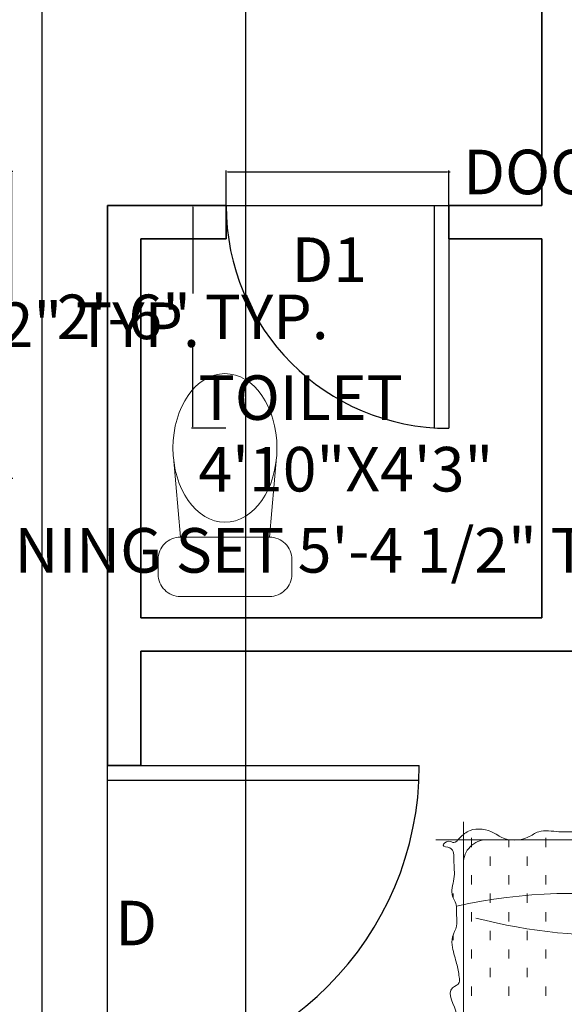
# Model space of a CAD drawing. Units: inches. Extents: x -26 to 575, y -18 to 513.
# Tile 8 of 28: x 122 to 196, y 191 to 324. Entities that reach past the tile are written whole.
import ezdxf

# ---------------------------------------------------------------- set-up
doc = ezdxf.new("R2010")
doc.units = ezdxf.units.IN
doc.header["$MEASUREMENT"] = 0
for name, color, linetype, lineweight in [('A-ANNO-DIMS', 2, 'Continuous', 18), ('A-ANNO-TEXT', 7, 'Continuous', 18), ('A-AREA-IDEN', 7, 'Continuous', 18), ('A-DOOR', 3, 'Continuous', 25), ('A-FLOR-FIXT', 9, 'Continuous', 18), ('A-WALL', 7, 'Continuous', 35), ('Furniture', 8, 'Continuous', 15)]:
    doc.layers.add(name, color=color, linetype=linetype, lineweight=lineweight)
doc.styles.get("Standard").update_dxf_attribs({"font": 'arial.ttf', "height": 6})
doc.dimstyles.get("Standard").update_dxf_attribs({"dimtxt": 6, "dimasz": 0.18, "dimexe": 0.18, "dimexo": 0.0625, "dimgap": 0.09, "dimtad": 0, "dimtih": 1, "dimtoh": 1, "dimzin": 0, "dimdsep": 46, "dimlunit": 3, "dimtxsty": 'Standard', "dimcen": 0.09, "dimadec": 0, "dimazin": 0, "dimtfac": 1, "dimtofl": 0, "dimtmove": 0, "dimatfit": 3, "dimfxl": 1, "dimtolj": 1, "dimtzin": 0, "dimarcsym": 0})

# ---------------------------------------------------------------- blocks, each defined once
blk = doc.blocks.new('BED-DOUBLE-WITH-NIGHTSTANDS')
for p, q in [((81.88, 42.36), (81.88, 0)), ((70.77, 22.17), (70.77, 23.42)), ((75.77, 22.17), (75.77, 23.42)), ((80.77, 22.17), (80.77, 23.42)), ((73.27, 19.67), (73.27, 20.92)), ((78.27, 19.67), (78.27, 20.92)), ((70.77, 17.17), (70.77, 18.42)), ((75.77, 17.17), (75.77, 18.42)), ((80.77, 17.17), (80.77, 18.42)), ((73.27, 14.67), (73.27, 15.92)), ((78.27, 14.67), (78.27, 15.92)), ((83.27, 15.26), (83.27, 15.92)), ((70.77, 12.17), (70.77, 13.42)), ((75.77, 12.17), (75.77, 13.42)), ((80.77, 12.17), (80.77, 13.42)), ((73.27, 9.67), (73.27, 10.92)), ((78.27, 9.67), (78.27, 10.92)), ((83.27, 9.67), (83.27, 10.2)), ((70.77, 7.17), (70.77, 8.42)), ((75.77, 7.17), (75.77, 8.42)), ((80.77, 7.17), (80.77, 8.42)), ((73.27, 4.67), (73.27, 5.92)), ((78.27, 4.67), (78.27, 5.92)), ((70.77, 2.17), (70.77, 3.42)), ((75.77, 2.41), (75.77, 3.42)), ((80.77, 2.17), (80.77, 3.42)), ((85.58, 2.43), (23.7, 2.43))]:
    blk.add_line(p, q)
for centre, radius, start, end in [((66.97, 82.6), 72.97, 239.8126, 282.5472), ((61.48, -60.53), 75.85, 75.7143, 109.4459), ((78.73, 5.58), 3.15, 270, 0)]:
    blk.add_arc(centre, radius, start, end)
blk.add_open_spline([(82.95, 38.85), (82.91, 38.17), (82.85, 36.97), (81.76, 35.43), (82.66, 33.92), (82.17, 32.16), (83.17, 30.81), (83.54, 28.6), (81.84, 26.13), (84.59, 22.62), (82.27, 21.86), (82.5, 20.48), (82.77, 18.98), (83.36, 17.21), (83.5, 15.41), (82.61, 14.09), (82.87, 12.46), (82.71, 11.04), (83.72, 9.61), (82.91, 7.55), (83.23, 5.58), (83.08, 3.39), (85.08, 3.34), (83.88, 2.36), (83.09, 3.04), (82.19, 1.93), (80.71, 0.69), (78.27, 1.05), (76.16, 2.63), (73.68, 2.58), (71.48, 0.95), (69.05, 1.47), (65.15, 1.19), (60.81, 2), (56.05, 2.59), (52.45, 0.27), (49.19, 1.51), (46.12, 1.7), (37.69, 3.67), (31.84, 3.18), (20.44, -0.09), (22.21, 3.75), (19.18, -0.44), (22.91, 0.39), (27.14, 0.63), (21.63, 1.85), (19.68, 4.27), (19.87, 11.16), (24.26, 3.84), (20.3, 10.76), (23.26, 12.85), (24.33, 17.43), (16.78, 17.59), (25.96, 19.23), (16.2, 20.68), (24.67, 22.01), (20.04, 24.96), (24.6, 28.15), (20.03, 29.6), (23.48, 31.6), (22.43, 34.55), (22.92, 41.18), (22.85, 37.06), (22.83, 35.35)], degree=3, knots=[0, 0, 0, 0, 2.033881, 3.581387, 5.07489, 6.704853, 8.655612, 9.757262, 13.24098, 16.903694, 18.063816, 18.788243, 20.635227, 22.875483, 24.324336, 25.871843, 27.320698, 29.140811, 29.950855, 32.312207, 34.847704, 36.565952, 37.541804, 38.447727, 39.194923, 40.100844, 41.912688, 45.194843, 46.251388, 49.875946, 51.496686, 54.215105, 56.7523, 63.316606, 67.484853, 70.581422, 75.324573, 76.965649, 79.915763, 100.671038, 102.483321, 104.317501, 106.523635, 109.038061, 111.571263, 115.809372, 117.667229, 122.411431, 125.445794, 129.976907, 132.758854, 136.424739, 139.918708, 143.481583, 147.135325, 151.002466, 153.252794, 157.23352, 159.244583, 161.905351, 164.097269, 169.015093, 172.531686, 172.531686, 172.531686, 172.531686])
blk = doc.blocks.new('DOOR-SWING-42IN')
for p, q in [((0, 0), (0, 42)), ((2, 0), (2, 42)), ((42, 0), (0, 0))]:
    blk.add_line(p, q)
blk.add_arc((0, 0), 42, 0, 90)
blk = doc.blocks.new('DOOR-SWING-30IN')
for p, q in [((-30, 0), (0, 0)), ((-2, 0), (-2, -30)), ((0, 0), (0, -30))]:
    blk.add_line(p, q)
blk.add_arc((0, 0), 30, 180, 270)
blk = doc.blocks.new('WC-FLOOR-MOUNT')
for p, q in [((-6, 8), (-6.95, 18.75)), ((6, 8), (6.95, 18.75))]:
    blk.add_line(p, q)
blk.add_lwpolyline([(-6, 8), (6, 8, -0.414214), (9, 5), (9, 3, -0.414214), (6, 0), (-6, 0, -0.414214), (-9, 3), (-9, 5, -0.414214)], format="xyb", close=True)
blk.add_ellipse((0, 20), major_axis=(0, 10), ratio=0.7)
blk = doc.blocks.new('*D16')
at = {"layer": 'A-ANNO-DIMS', "color": 0, "lineweight": -2, "transparency": 16777216}
for p, q in [((150.16, 298.57), (150.16, 303.19)), ((150.34, 303.01), (179.98, 303.01)), ((180.16, 298.57), (180.16, 303.19)), ((180.16, 303.01), (180.34, 303.01))]:
    blk.add_line(p, q, dxfattribs=at)
at = {"layer": 'A-ANNO-DIMS', "color": 0, "transparency": 16777216}
for points in [[(150.34, 303.04), (150.34, 302.98), (150.16, 303.01)], [(179.98, 303.04), (179.98, 302.98), (180.16, 303.01)]]:
    blk.add_solid(points, dxfattribs=at)
at = {"layer": 'Defpoints', "color": 0, "transparency": 16777216}
for p in [(180.16, 303.01), (150.16, 298.51), (180.16, 298.51)]:
    blk.add_point(p, dxfattribs=at)
at = {"layer": 'A-ANNO-DIMS', "color": 0, "transparency": 16777216, "insert": (218.82, 303.01), "char_height": 6, "attachment_point": 5}
blk.add_mtext('\\A1;DOOR D1 2\'-6" TYP.', dxfattribs=at)
blk = doc.blocks.new('*D17')
at = {"layer": 'A-ANNO-DIMS', "color": 0, "lineweight": -2, "transparency": 16777216}
for p, q in [((150.1, 298.51), (145.48, 298.51)), ((145.66, 298.33), (145.66, 286.66)), ((145.66, 268.69), (145.66, 280.35)), ((150.1, 268.51), (145.48, 268.51))]:
    blk.add_line(p, q, dxfattribs=at)
at = {"layer": 'A-ANNO-DIMS', "color": 0, "transparency": 16777216}
for points in [[(145.63, 298.33), (145.69, 298.33), (145.66, 298.51)], [(145.63, 268.69), (145.69, 268.69), (145.66, 268.51)]]:
    blk.add_solid(points, dxfattribs=at)
at = {"layer": 'Defpoints', "color": 0, "transparency": 16777216}
for p in [(145.66, 298.51), (150.16, 298.51), (150.16, 268.51)]:
    blk.add_point(p, dxfattribs=at)
at = {"layer": 'A-ANNO-DIMS', "color": 0, "transparency": 16777216, "insert": (145.66, 283.51), "char_height": 6, "attachment_point": 5}
blk.add_mtext('\\A1;2\'-6" TYP.', dxfattribs=at)
blk = doc.blocks.new('*D24')
at = {"layer": 'A-ANNO-DIMS', "color": 0, "lineweight": -2, "transparency": 16777216}
for p, q in [((46.82, 261.72), (46.82, 251.9)), ((111.54, 261.72), (111.54, 251.9)), ((47, 252.08), (111.36, 252.08)), ((111.54, 252.08), (111.72, 252.08))]:
    blk.add_line(p, q, dxfattribs=at)
at = {"layer": 'A-ANNO-DIMS', "color": 0, "transparency": 16777216}
for points in [[(47, 252.11), (47, 252.05), (46.82, 252.08)], [(111.36, 252.11), (111.36, 252.05), (111.54, 252.08)]]:
    blk.add_solid(points, dxfattribs=at)
at = {"layer": 'Defpoints', "color": 0, "transparency": 16777216}
for p in [(46.82, 261.79), (111.54, 261.79), (111.54, 252.08)]:
    blk.add_point(p, dxfattribs=at)
at = {"layer": 'A-ANNO-DIMS', "color": 0, "transparency": 16777216, "insert": (162.09, 252.08), "char_height": 6, "attachment_point": 5}
blk.add_mtext('\\A1;DINING SET 5\'-4 1/2" TYP.', dxfattribs=at)
blk = doc.blocks.new('*D25')
at = {"layer": 'A-ANNO-DIMS', "color": 0, "lineweight": -2, "transparency": 16777216}
for p, q in [((111.61, 303.12), (121.43, 303.12)), ((121.25, 302.94), (121.25, 285.65)), ((121.25, 261.97), (121.25, 279.26)), ((111.61, 261.79), (121.43, 261.79))]:
    blk.add_line(p, q, dxfattribs=at)
at = {"layer": 'A-ANNO-DIMS', "color": 0, "transparency": 16777216}
for points in [[(121.22, 302.94), (121.28, 302.94), (121.25, 303.12)], [(121.22, 261.97), (121.28, 261.97), (121.25, 261.79)]]:
    blk.add_solid(points, dxfattribs=at)
at = {"layer": 'Defpoints', "color": 0, "transparency": 16777216}
for p in [(111.54, 303.12), (121.25, 303.12), (111.54, 261.79)]:
    blk.add_point(p, dxfattribs=at)
at = {"layer": 'A-ANNO-DIMS', "color": 0, "transparency": 16777216, "insert": (121.25, 282.45), "char_height": 6, "attachment_point": 5}
blk.add_mtext('\\A1;3\'-5 1/2" TYP.', dxfattribs=at)
blk = doc.blocks.new('*D29')
at = {"layer": 'A-ANNO-DIMS', "color": 0, "lineweight": -2, "transparency": 16777216}
for p, q in [((125.35, 466.45), (125.35, -8.97)), ((152.78, 466.45), (152.78, -8.97)), ((125.53, -8.79), (152.6, -8.79)), ((152.78, -8.79), (152.96, -8.79))]:
    blk.add_line(p, q, dxfattribs=at)
at = {"layer": 'A-ANNO-DIMS', "color": 0, "transparency": 16777216}
for points in [[(125.53, -8.76), (125.53, -8.82), (125.35, -8.79)], [(152.6, -8.76), (152.6, -8.82), (152.78, -8.79)]]:
    blk.add_solid(points, dxfattribs=at)
at = {"layer": 'Defpoints', "color": 0, "transparency": 16777216}
for p in [(125.35, 466.51), (152.78, 466.51), (152.78, -8.79)]:
    blk.add_point(p, dxfattribs=at)
at = {"layer": 'A-ANNO-DIMS', "color": 0, "transparency": 16777216, "insert": (168.07, -8.79), "char_height": 6, "attachment_point": 5}
blk.add_mtext('\\A1;2\'-3 1/2"', dxfattribs=at)

msp = doc.modelspace()

# ---------------------------------------------------------------- linework, layer by layer
at = {"layer": 'A-WALL'}
for p, q in [((192.677, 298.508), (192.677, 330.008)), ((134.177, 223.131), (134.177, 298.508)), ((150.159, 298.508), (134.177, 298.508)), ((150.159, 298.508), (150.159, 294.008)), ((192.677, 298.508), (180.159, 298.508)), ((180.159, 298.508), (180.159, 294.008)), ((138.677, 243.008), (138.677, 294.008)), ((150.159, 294.008), (138.677, 294.008)), ((192.677, 294.008), (180.159, 294.008)), ((192.677, 243.008), (192.677, 294.008)), ((192.677, 243.008), (138.677, 243.008)), ((269.177, 238.508), (138.677, 238.508)), ((138.677, 223.131), (138.677, 238.508)), ((134.177, 223.131), (138.677, 223.131))]:
    msp.add_line(p, q, dxfattribs=at)

# ---------------------------------------------------------------- block references
at = {"layer": 'A-DOOR'}
msp.add_blockref('DOOR-SWING-30IN', (180.159, 298.508), dxfattribs=at)
at = {"layer": 'A-DOOR', "rotation": 269.9999999999999}
msp.add_blockref('DOOR-SWING-42IN', (134.177, 223.131), dxfattribs=at)
at = {"layer": 'A-FLOR-FIXT'}
msp.add_blockref('WC-FLOOR-MOUNT', (150.004, 245.867), dxfattribs=at)
at = {"layer": 'Furniture', "rotation": 180}
msp.add_blockref('BED-DOUBLE-WITH-NIGHTSTANDS', (263.993, 215.545), dxfattribs=at)

# ---------------------------------------------------------------- texts
at = {"layer": 'A-ANNO-TEXT'}
for s, p in [('D1', (158.959, 288.207)), ('D', (135.225, 198.912))]:
    msp.add_text(s, height=6, rotation=0.00167, dxfattribs=at).set_placement(p)
at = {"layer": 'A-AREA-IDEN'}
for s, p in [('TOILET', (146.427, 269.641)), ('4\'10"X4\'3"', (146.427, 260.003))]:
    msp.add_text(s, height=6, rotation=0.00167, dxfattribs=at).set_placement(p)

# ---------------------------------------------------------------- dimensions: what is measured, and where the dimension line sits
at = {"layer": 'A-ANNO-DIMS'}
dim = msp.add_linear_dim(base=(152.784, -8.792), p1=(125.349, 466.508), p2=(152.784, 466.508), dimstyle='Standard', override={"dimdec": 1, "dimlfac": 1, "dimrnd": 0, "dimzin": 1, "dimdsep": 46, "dimlunit": 4, "dimfrac": 2}, dxfattribs=at)
dim.commit()
dim.dimension.update_dxf_attribs({"geometry": '*D29', "text_midpoint": (168.07, -8.792)})
for base, p1, p2, text, picture, middle in [((180.159, 303.008), (150.159, 298.508), (180.159, 298.508), 'DOOR D1 <> TYP.', '*D16', (218.825, 303.008)), ((111.544, 252.079), (46.82, 261.787), (111.544, 261.787), 'DINING SET <> TYP.', '*D24', (162.09, 252.079))]:
    dim = msp.add_linear_dim(base=base, p1=p1, p2=p2, text=text, dimstyle='Standard', override={"dimdec": 1, "dimlfac": 1, "dimrnd": 0, "dimzin": 1, "dimdsep": 46, "dimlunit": 4, "dimfrac": 2}, dxfattribs=at)
    dim.commit()
    dim.dimension.update_dxf_attribs({"geometry": picture, "text_midpoint": middle})
for base, p1, p2, picture, middle in [((121.253, 303.116), (111.544, 261.787), (111.544, 303.116), '*D25', (121.253, 282.452)), ((145.659, 298.508), (150.159, 268.508), (150.159, 298.508), '*D17', (145.659, 283.508))]:
    dim = msp.add_linear_dim(base=base, p1=p1, p2=p2, angle=90, text='<> TYP.', dimstyle='Standard', override={"dimdec": 1, "dimlfac": 1, "dimrnd": 0, "dimzin": 1, "dimdsep": 46, "dimlunit": 4, "dimfrac": 2}, dxfattribs=at)
    dim.commit()
    dim.dimension.update_dxf_attribs({"geometry": picture, "text_midpoint": middle})

doc.saveas('drawing.dxf')
